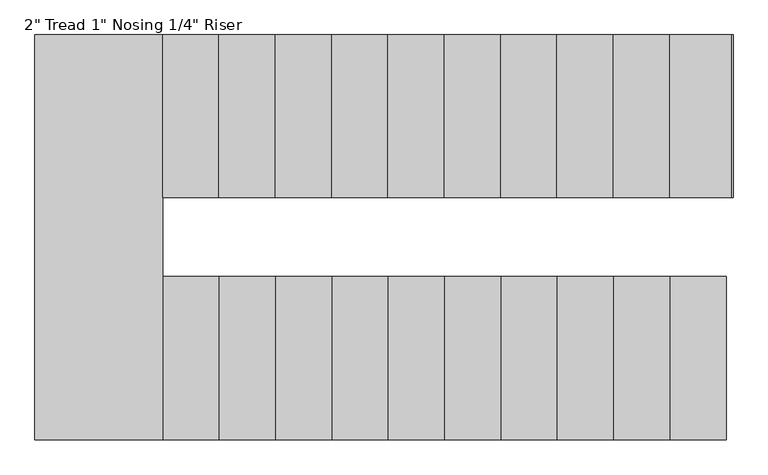
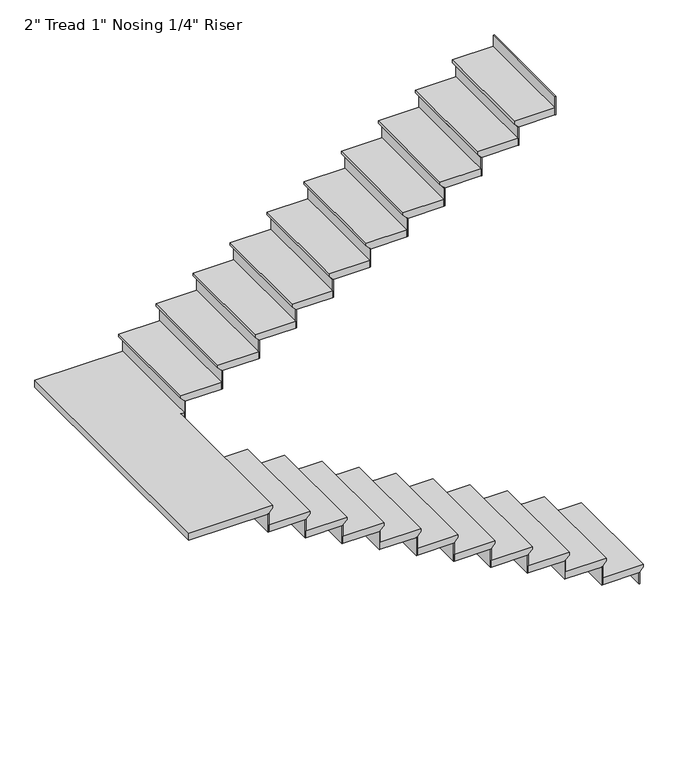
"""IFC4 building model written with IfcOpenShell, lengths in millimetres: stair flight geometry."""

from ifc_helpers import new_model, si_unit, origin, place, context, project, spatial, faceted_brep, source, transform, mapped, element, save


def stair_flight_f3bed003(model_context):
    return source(origin(), model_context, "Body", "Brep", [
        faceted_brep([(-3117.2664982, -6914.3822004, 112.5681818), (-3117.2664982, -6914.3822004, 131.6181818), (-3117.2664982, -7650.9822004, 131.6181818), (-3117.2664982, -7650.9822004, 112.5681818), (-3142.6664982, -6914.3822004, 87.1681818), (-3142.6664982, -7650.9822004, 87.1681818), (-3396.6664982, -6914.3822004, 131.6181818), (-3396.6664982, -7650.9822004, 131.6181818), (-3142.6664982, -7650.9822004, 80.8181818), (-3396.6664982, -7650.9822004, 80.8181818), (-3396.6664982, -6914.3822004, 80.8181818), (-3142.6664982, -6914.3822004, 80.8181818)], [[[0, 1, 2, 3]], [[4, 0, 3, 5]], [[2, 1, 6, 7]], [[8, 9, 10, 11]], [[2, 7, 9, 8, 5, 3]], [[8, 11, 4, 5]], [[6, 1, 0, 4, 11, 10]], [[7, 6, 10, 9]]]),
        faceted_brep([(-3142.6664982, -6914.3822004, 80.8181818), (-3142.6664982, -6914.3822004, 0.0), (-3149.0164982, -6914.3822004, 0.0), (-3149.0164982, -6914.3822004, 80.8181818), (-3142.6664982, -7650.9822004, 80.8181818), (-3149.0164982, -7650.9822004, 80.8181818), (-3149.0164982, -7650.9822004, 0.0), (-3142.6664982, -7650.9822004, 0.0)], [[[0, 1, 2, 3]], [[4, 5, 6, 7]], [[1, 0, 4, 7]], [[2, 1, 7, 6]], [[3, 2, 6, 5]], [[0, 3, 5, 4]]]),
        faceted_brep([(-3396.6664982, -6914.3822004, 212.4363636), (-3396.6664982, -6914.3822004, 80.8181818), (-3403.0164982, -6914.3822004, 80.8181818), (-3403.0164982, -6914.3822004, 212.4363636), (-3396.6664982, -7650.9822004, 212.4363636), (-3403.0164982, -7650.9822004, 212.4363636), (-3403.0164982, -7650.9822004, 80.8181818), (-3396.6664982, -7650.9822004, 80.8181818)], [[[0, 1, 2, 3]], [[4, 5, 6, 7]], [[1, 0, 4, 7]], [[2, 1, 7, 6]], [[3, 2, 6, 5]], [[0, 3, 5, 4]]]),
        faceted_brep([(-3371.2664982, -7650.9822004, 263.2363636), (-3371.2664982, -6914.3822004, 263.2363636), (-3650.6664982, -6914.3822004, 263.2363636), (-3650.6664982, -7650.9822004, 263.2363636), (-3396.6664982, -7650.9822004, 212.4363636), (-3650.6664982, -7650.9822004, 212.4363636), (-3650.6664982, -6914.3822004, 212.4363636), (-3396.6664982, -6914.3822004, 212.4363636), (-3396.6664982, -7650.9822004, 218.7863636), (-3371.2664982, -7650.9822004, 244.1863636), (-3396.6664982, -6914.3822004, 218.7863636), (-3371.2664982, -6914.3822004, 244.1863636)], [[[0, 1, 2, 3]], [[4, 5, 6, 7]], [[0, 3, 5, 4, 8, 9]], [[4, 7, 10, 8]], [[2, 1, 11, 10, 7, 6]], [[3, 2, 6, 5]], [[11, 1, 0, 9]], [[10, 11, 9, 8]]]),
        faceted_brep([(-3650.6664982, -6914.3822004, 344.0545455), (-3650.6664982, -6914.3822004, 212.4363636), (-3657.0164982, -6914.3822004, 212.4363636), (-3657.0164982, -6914.3822004, 344.0545455), (-3650.6664982, -7650.9822004, 344.0545455), (-3657.0164982, -7650.9822004, 344.0545455), (-3657.0164982, -7650.9822004, 212.4363636), (-3650.6664982, -7650.9822004, 212.4363636)], [[[0, 1, 2, 3]], [[4, 5, 6, 7]], [[1, 0, 4, 7]], [[2, 1, 7, 6]], [[3, 2, 6, 5]], [[0, 3, 5, 4]]]),
        faceted_brep([(-3625.2664982, -7650.9822004, 394.8545455), (-3625.2664982, -6914.3822004, 394.8545455), (-3904.6664982, -6914.3822004, 394.8545455), (-3904.6664982, -7650.9822004, 394.8545455), (-3650.6664982, -7650.9822004, 344.0545455), (-3904.6664982, -7650.9822004, 344.0545455), (-3904.6664982, -6914.3822004, 344.0545455), (-3650.6664982, -6914.3822004, 344.0545455), (-3650.6664982, -7650.9822004, 350.4045455), (-3625.2664982, -7650.9822004, 375.8045455), (-3650.6664982, -6914.3822004, 350.4045455), (-3625.2664982, -6914.3822004, 375.8045455)], [[[0, 1, 2, 3]], [[4, 5, 6, 7]], [[0, 3, 5, 4, 8, 9]], [[4, 7, 10, 8]], [[2, 1, 11, 10, 7, 6]], [[3, 2, 6, 5]], [[11, 1, 0, 9]], [[10, 11, 9, 8]]]),
        faceted_brep([(-3904.6664982, -6914.3822004, 475.6727273), (-3904.6664982, -6914.3822004, 344.0545455), (-3911.0164982, -6914.3822004, 344.0545455), (-3911.0164982, -6914.3822004, 475.6727273), (-3904.6664982, -7650.9822004, 475.6727273), (-3911.0164982, -7650.9822004, 475.6727273), (-3911.0164982, -7650.9822004, 344.0545455), (-3904.6664982, -7650.9822004, 344.0545455)], [[[0, 1, 2, 3]], [[4, 5, 6, 7]], [[1, 0, 4, 7]], [[2, 1, 7, 6]], [[3, 2, 6, 5]], [[0, 3, 5, 4]]]),
        faceted_brep([(-3879.2664982, -7650.9822004, 526.4727273), (-3879.2664982, -6914.3822004, 526.4727273), (-4158.6664982, -6914.3822004, 526.4727273), (-4158.6664982, -7650.9822004, 526.4727273), (-3904.6664982, -7650.9822004, 475.6727273), (-4158.6664982, -7650.9822004, 475.6727273), (-4158.6664982, -6914.3822004, 475.6727273), (-3904.6664982, -6914.3822004, 475.6727273), (-3904.6664982, -7650.9822004, 482.0227273), (-3879.2664982, -7650.9822004, 507.4227273), (-3904.6664982, -6914.3822004, 482.0227273), (-3879.2664982, -6914.3822004, 507.4227273)], [[[0, 1, 2, 3]], [[4, 5, 6, 7]], [[0, 3, 5, 4, 8, 9]], [[4, 7, 10, 8]], [[2, 1, 11, 10, 7, 6]], [[3, 2, 6, 5]], [[11, 1, 0, 9]], [[10, 11, 9, 8]]]),
        faceted_brep([(-4158.6664982, -6914.3822004, 607.2909091), (-4158.6664982, -6914.3822004, 475.6727273), (-4165.0164982, -6914.3822004, 475.6727273), (-4165.0164982, -6914.3822004, 607.2909091), (-4158.6664982, -7650.9822004, 607.2909091), (-4165.0164982, -7650.9822004, 607.2909091), (-4165.0164982, -7650.9822004, 475.6727273), (-4158.6664982, -7650.9822004, 475.6727273)], [[[0, 1, 2, 3]], [[4, 5, 6, 7]], [[1, 0, 4, 7]], [[2, 1, 7, 6]], [[3, 2, 6, 5]], [[0, 3, 5, 4]]]),
        faceted_brep([(-4133.2664982, -7650.9822004, 658.0909091), (-4133.2664982, -6914.3822004, 658.0909091), (-4412.6664982, -6914.3822004, 658.0909091), (-4412.6664982, -7650.9822004, 658.0909091), (-4158.6664982, -7650.9822004, 607.2909091), (-4412.6664982, -7650.9822004, 607.2909091), (-4412.6664982, -6914.3822004, 607.2909091), (-4158.6664982, -6914.3822004, 607.2909091), (-4158.6664982, -7650.9822004, 613.6409091), (-4133.2664982, -7650.9822004, 639.0409091), (-4158.6664982, -6914.3822004, 613.6409091), (-4133.2664982, -6914.3822004, 639.0409091)], [[[0, 1, 2, 3]], [[4, 5, 6, 7]], [[0, 3, 5, 4, 8, 9]], [[4, 7, 10, 8]], [[2, 1, 11, 10, 7, 6]], [[3, 2, 6, 5]], [[11, 1, 0, 9]], [[10, 11, 9, 8]]]),
        faceted_brep([(-4412.6664982, -6914.3822004, 738.9090909), (-4412.6664982, -6914.3822004, 607.2909091), (-4419.0164982, -6914.3822004, 607.2909091), (-4419.0164982, -6914.3822004, 738.9090909), (-4412.6664982, -7650.9822004, 738.9090909), (-4419.0164982, -7650.9822004, 738.9090909), (-4419.0164982, -7650.9822004, 607.2909091), (-4412.6664982, -7650.9822004, 607.2909091)], [[[0, 1, 2, 3]], [[4, 5, 6, 7]], [[1, 0, 4, 7]], [[2, 1, 7, 6]], [[3, 2, 6, 5]], [[0, 3, 5, 4]]]),
        faceted_brep([(-4387.2664982, -7650.9822004, 789.7090909), (-4387.2664982, -6914.3822004, 789.7090909), (-4666.6664982, -6914.3822004, 789.7090909), (-4666.6664982, -7650.9822004, 789.7090909), (-4412.6664982, -7650.9822004, 738.9090909), (-4666.6664982, -7650.9822004, 738.9090909), (-4666.6664982, -6914.3822004, 738.9090909), (-4412.6664982, -6914.3822004, 738.9090909), (-4412.6664982, -7650.9822004, 745.2590909), (-4387.2664982, -7650.9822004, 770.6590909), (-4412.6664982, -6914.3822004, 745.2590909), (-4387.2664982, -6914.3822004, 770.6590909)], [[[0, 1, 2, 3]], [[4, 5, 6, 7]], [[0, 3, 5, 4, 8, 9]], [[4, 7, 10, 8]], [[2, 1, 11, 10, 7, 6]], [[3, 2, 6, 5]], [[11, 1, 0, 9]], [[10, 11, 9, 8]]]),
        faceted_brep([(-4666.6664982, -6914.3822004, 870.5272727), (-4666.6664982, -6914.3822004, 738.9090909), (-4673.0164982, -6914.3822004, 738.9090909), (-4673.0164982, -6914.3822004, 870.5272727), (-4666.6664982, -7650.9822004, 870.5272727), (-4673.0164982, -7650.9822004, 870.5272727), (-4673.0164982, -7650.9822004, 738.9090909), (-4666.6664982, -7650.9822004, 738.9090909)], [[[0, 1, 2, 3]], [[4, 5, 6, 7]], [[1, 0, 4, 7]], [[2, 1, 7, 6]], [[3, 2, 6, 5]], [[0, 3, 5, 4]]]),
        faceted_brep([(-4641.2664982, -7650.9822004, 921.3272727), (-4641.2664982, -6914.3822004, 921.3272727), (-4920.6664982, -6914.3822004, 921.3272727), (-4920.6664982, -7650.9822004, 921.3272727), (-4666.6664982, -7650.9822004, 870.5272727), (-4920.6664982, -7650.9822004, 870.5272727), (-4920.6664982, -6914.3822004, 870.5272727), (-4666.6664982, -6914.3822004, 870.5272727), (-4666.6664982, -7650.9822004, 876.8772727), (-4641.2664982, -7650.9822004, 902.2772727), (-4666.6664982, -6914.3822004, 876.8772727), (-4641.2664982, -6914.3822004, 902.2772727)], [[[0, 1, 2, 3]], [[4, 5, 6, 7]], [[0, 3, 5, 4, 8, 9]], [[4, 7, 10, 8]], [[2, 1, 11, 10, 7, 6]], [[3, 2, 6, 5]], [[11, 1, 0, 9]], [[10, 11, 9, 8]]]),
        faceted_brep([(-4920.6664982, -6914.3822004, 1002.1454545), (-4920.6664982, -6914.3822004, 870.5272727), (-4927.0164982, -6914.3822004, 870.5272727), (-4927.0164982, -6914.3822004, 1002.1454545), (-4920.6664982, -7650.9822004, 1002.1454545), (-4927.0164982, -7650.9822004, 1002.1454545), (-4927.0164982, -7650.9822004, 870.5272727), (-4920.6664982, -7650.9822004, 870.5272727)], [[[0, 1, 2, 3]], [[4, 5, 6, 7]], [[1, 0, 4, 7]], [[2, 1, 7, 6]], [[3, 2, 6, 5]], [[0, 3, 5, 4]]]),
        faceted_brep([(-4895.2664982, -7650.9822004, 1052.9454545), (-4895.2664982, -6914.3822004, 1052.9454545), (-5174.6664982, -6914.3822004, 1052.9454545), (-5174.6664982, -7650.9822004, 1052.9454545), (-4920.6664982, -7650.9822004, 1002.1454545), (-5174.6664982, -7650.9822004, 1002.1454545), (-5174.6664982, -6914.3822004, 1002.1454545), (-4920.6664982, -6914.3822004, 1002.1454545), (-4920.6664982, -7650.9822004, 1008.4954545), (-4895.2664982, -7650.9822004, 1033.8954545), (-4920.6664982, -6914.3822004, 1008.4954545), (-4895.2664982, -6914.3822004, 1033.8954545)], [[[0, 1, 2, 3]], [[4, 5, 6, 7]], [[0, 3, 5, 4, 8, 9]], [[4, 7, 10, 8]], [[2, 1, 11, 10, 7, 6]], [[3, 2, 6, 5]], [[11, 1, 0, 9]], [[10, 11, 9, 8]]]),
        faceted_brep([(-5174.6664982, -6914.3822004, 1133.7636364), (-5174.6664982, -6914.3822004, 1002.1454545), (-5181.0164982, -6914.3822004, 1002.1454545), (-5181.0164982, -6914.3822004, 1133.7636364), (-5174.6664982, -7650.9822004, 1133.7636364), (-5181.0164982, -7650.9822004, 1133.7636364), (-5181.0164982, -7650.9822004, 1002.1454545), (-5174.6664982, -7650.9822004, 1002.1454545)], [[[0, 1, 2, 3]], [[4, 5, 6, 7]], [[1, 0, 4, 7]], [[2, 1, 7, 6]], [[3, 2, 6, 5]], [[0, 3, 5, 4]]]),
        faceted_brep([(-5149.2664982, -7650.9822004, 1184.5636364), (-5149.2664982, -6914.3822004, 1184.5636364), (-5428.6664982, -6914.3822004, 1184.5636364), (-5428.6664982, -7650.9822004, 1184.5636364), (-5174.6664982, -7650.9822004, 1133.7636364), (-5428.6664982, -7650.9822004, 1133.7636364), (-5428.6664982, -6914.3822004, 1133.7636364), (-5174.6664982, -6914.3822004, 1133.7636364), (-5174.6664982, -7650.9822004, 1140.1136364), (-5149.2664982, -7650.9822004, 1165.5136364), (-5174.6664982, -6914.3822004, 1140.1136364), (-5149.2664982, -6914.3822004, 1165.5136364)], [[[0, 1, 2, 3]], [[4, 5, 6, 7]], [[0, 3, 5, 4, 8, 9]], [[4, 7, 10, 8]], [[2, 1, 11, 10, 7, 6]], [[3, 2, 6, 5]], [[11, 1, 0, 9]], [[10, 11, 9, 8]]]),
        faceted_brep([(-5428.6664982, -6914.3822004, 1265.3818182), (-5428.6664982, -6914.3822004, 1133.7636364), (-5435.0164982, -6914.3822004, 1133.7636364), (-5435.0164982, -6914.3822004, 1265.3818182), (-5428.6664982, -7650.9822004, 1265.3818182), (-5435.0164982, -7650.9822004, 1265.3818182), (-5435.0164982, -7650.9822004, 1133.7636364), (-5428.6664982, -7650.9822004, 1133.7636364)], [[[0, 1, 2, 3]], [[4, 5, 6, 7]], [[1, 0, 4, 7]], [[2, 1, 7, 6]], [[3, 2, 6, 5]], [[0, 3, 5, 4]]]),
        faceted_brep([(-5403.2664982, -7650.9822004, 1316.1818182), (-5403.2664982, -6914.3822004, 1316.1818182), (-5682.6664982, -6914.3822004, 1316.1818182), (-5682.6664982, -7650.9822004, 1316.1818182), (-5428.6664982, -7650.9822004, 1265.3818182), (-5682.6664982, -7650.9822004, 1265.3818182), (-5682.6664982, -6914.3822004, 1265.3818182), (-5428.6664982, -6914.3822004, 1265.3818182), (-5428.6664982, -7650.9822004, 1271.7318182), (-5403.2664982, -7650.9822004, 1297.1318182), (-5428.6664982, -6914.3822004, 1271.7318182), (-5403.2664982, -6914.3822004, 1297.1318182)], [[[0, 1, 2, 3]], [[4, 5, 6, 7]], [[0, 3, 5, 4, 8, 9]], [[4, 7, 10, 8]], [[2, 1, 11, 10, 7, 6]], [[3, 2, 6, 5]], [[11, 1, 0, 9]], [[10, 11, 9, 8]]]),
        faceted_brep([(-5682.6664982, -6914.3822004, 1397.0), (-5682.6664982, -6914.3822004, 1265.3818182), (-5689.0164982, -6914.3822004, 1265.3818182), (-5689.0164982, -6914.3822004, 1397.0), (-5682.6664982, -7650.9822004, 1397.0), (-5689.0164982, -7650.9822004, 1397.0), (-5689.0164982, -7650.9822004, 1265.3818182), (-5682.6664982, -7650.9822004, 1265.3818182)], [[[0, 1, 2, 3]], [[4, 5, 6, 7]], [[1, 0, 4, 7]], [[2, 1, 7, 6]], [[3, 2, 6, 5]], [[0, 3, 5, 4]]]),
        faceted_brep([(-5631.8664982, -5824.7082131, 1447.8), (-6232.5131972, -5824.7082131, 1447.8), (-6232.5131972, -7650.9822004, 1447.8), (-5657.2664982, -7650.9822004, 1447.8), (-5657.2664982, -6558.7822004, 1447.8), (-5631.8664982, -6558.7822004, 1447.8), (-6232.5131972, -5824.7082131, 1397.0), (-5631.8664982, -5824.7082131, 1397.0), (-5631.8664982, -6558.7822004, 1397.0), (-5657.2664982, -6558.7822004, 1397.0), (-5657.2664982, -6914.3822004, 1397.0), (-5682.6664982, -6914.3822004, 1397.0), (-5682.6664982, -7650.9822004, 1397.0), (-6232.5131972, -7650.9822004, 1397.0), (-5682.6664982, -6914.3822004, 1403.35), (-5682.6664982, -7650.9822004, 1403.35), (-5657.2664982, -7650.9822004, 1428.75), (-5657.2664982, -6914.3822004, 1428.75)], [[[0, 1, 2, 3, 4, 5]], [[6, 7, 8, 9, 10, 11, 12, 13]], [[1, 0, 7, 6]], [[2, 1, 6, 13]], [[12, 11, 14, 15]], [[4, 3, 16, 17, 10, 9]], [[5, 4, 9, 8]], [[0, 5, 8, 7]], [[16, 15, 14, 17]], [[3, 2, 13, 12, 15, 16]], [[11, 10, 17, 14]]]),
        faceted_brep([(-5631.8664982, -6558.7822004, 1528.6181818), (-5631.8664982, -6558.7822004, 1397.0), (-5625.5164982, -6558.7822004, 1397.0), (-5625.5164982, -6558.7822004, 1528.6181818), (-5631.8664982, -5824.7082131, 1528.6181818), (-5625.5164982, -5824.7082131, 1528.6181818), (-5625.5164982, -5824.7082131, 1397.0), (-5631.8664982, -5824.7082131, 1397.0)], [[[0, 1, 2, 3]], [[4, 5, 6, 7]], [[1, 0, 4, 7]], [[2, 1, 7, 6]], [[3, 2, 6, 5]], [[0, 3, 5, 4]]]),
        faceted_brep([(-5657.2664982, -5824.7082131, 1579.4181818), (-5657.2664982, -6558.7822004, 1579.4181818), (-5377.8664982, -6558.7822004, 1579.4181818), (-5377.8664982, -5824.7082131, 1579.4181818), (-5631.8664982, -5824.7082131, 1528.6181818), (-5377.8664982, -5824.7082131, 1528.6181818), (-5377.8664982, -6558.7822004, 1528.6181818), (-5631.8664982, -6558.7822004, 1528.6181818), (-5631.8664982, -5824.7082131, 1534.9681818), (-5657.2664982, -5824.7082131, 1560.3681818), (-5631.8664982, -6558.7822004, 1534.9681818), (-5657.2664982, -6558.7822004, 1560.3681818)], [[[0, 1, 2, 3]], [[4, 5, 6, 7]], [[0, 3, 5, 4, 8, 9]], [[4, 7, 10, 8]], [[2, 1, 11, 10, 7, 6]], [[3, 2, 6, 5]], [[11, 1, 0, 9]], [[10, 11, 9, 8]]]),
        faceted_brep([(-5377.8664982, -6558.7822004, 1660.2363636), (-5377.8664982, -6558.7822004, 1528.6181818), (-5371.5164982, -6558.7822004, 1528.6181818), (-5371.5164982, -6558.7822004, 1660.2363636), (-5377.8664982, -5824.7082131, 1660.2363636), (-5371.5164982, -5824.7082131, 1660.2363636), (-5371.5164982, -5824.7082131, 1528.6181818), (-5377.8664982, -5824.7082131, 1528.6181818)], [[[0, 1, 2, 3]], [[4, 5, 6, 7]], [[1, 0, 4, 7]], [[2, 1, 7, 6]], [[3, 2, 6, 5]], [[0, 3, 5, 4]]]),
        faceted_brep([(-5403.2664982, -5824.7082131, 1711.0363636), (-5403.2664982, -6558.7822004, 1711.0363636), (-5123.8664982, -6558.7822004, 1711.0363636), (-5123.8664982, -5824.7082131, 1711.0363636), (-5377.8664982, -5824.7082131, 1660.2363636), (-5123.8664982, -5824.7082131, 1660.2363636), (-5123.8664982, -6558.7822004, 1660.2363636), (-5377.8664982, -6558.7822004, 1660.2363636), (-5377.8664982, -5824.7082131, 1666.5863636), (-5403.2664982, -5824.7082131, 1691.9863636), (-5377.8664982, -6558.7822004, 1666.5863636), (-5403.2664982, -6558.7822004, 1691.9863636)], [[[0, 1, 2, 3]], [[4, 5, 6, 7]], [[0, 3, 5, 4, 8, 9]], [[4, 7, 10, 8]], [[2, 1, 11, 10, 7, 6]], [[3, 2, 6, 5]], [[11, 1, 0, 9]], [[10, 11, 9, 8]]]),
        faceted_brep([(-5123.8664982, -6558.7822004, 1791.8545455), (-5123.8664982, -6558.7822004, 1660.2363636), (-5117.5164982, -6558.7822004, 1660.2363636), (-5117.5164982, -6558.7822004, 1791.8545455), (-5123.8664982, -5824.7082131, 1791.8545455), (-5117.5164982, -5824.7082131, 1791.8545455), (-5117.5164982, -5824.7082131, 1660.2363636), (-5123.8664982, -5824.7082131, 1660.2363636)], [[[0, 1, 2, 3]], [[4, 5, 6, 7]], [[1, 0, 4, 7]], [[2, 1, 7, 6]], [[3, 2, 6, 5]], [[0, 3, 5, 4]]]),
        faceted_brep([(-5149.2664982, -5824.7082131, 1842.6545455), (-5149.2664982, -6558.7822004, 1842.6545455), (-4869.8664982, -6558.7822004, 1842.6545455), (-4869.8664982, -5824.7082131, 1842.6545455), (-5123.8664982, -5824.7082131, 1791.8545455), (-4869.8664982, -5824.7082131, 1791.8545455), (-4869.8664982, -6558.7822004, 1791.8545455), (-5123.8664982, -6558.7822004, 1791.8545455), (-5123.8664982, -5824.7082131, 1798.2045455), (-5149.2664982, -5824.7082131, 1823.6045455), (-5123.8664982, -6558.7822004, 1798.2045455), (-5149.2664982, -6558.7822004, 1823.6045455)], [[[0, 1, 2, 3]], [[4, 5, 6, 7]], [[0, 3, 5, 4, 8, 9]], [[4, 7, 10, 8]], [[2, 1, 11, 10, 7, 6]], [[3, 2, 6, 5]], [[11, 1, 0, 9]], [[10, 11, 9, 8]]]),
        faceted_brep([(-4869.8664982, -6558.7822004, 1923.4727273), (-4869.8664982, -6558.7822004, 1791.8545455), (-4863.5164982, -6558.7822004, 1791.8545455), (-4863.5164982, -6558.7822004, 1923.4727273), (-4869.8664982, -5824.7082131, 1923.4727273), (-4863.5164982, -5824.7082131, 1923.4727273), (-4863.5164982, -5824.7082131, 1791.8545455), (-4869.8664982, -5824.7082131, 1791.8545455)], [[[0, 1, 2, 3]], [[4, 5, 6, 7]], [[1, 0, 4, 7]], [[2, 1, 7, 6]], [[3, 2, 6, 5]], [[0, 3, 5, 4]]]),
        faceted_brep([(-4895.2664982, -5824.7082131, 1974.2727273), (-4895.2664982, -6558.7822004, 1974.2727273), (-4615.8664982, -6558.7822004, 1974.2727273), (-4615.8664982, -5824.7082131, 1974.2727273), (-4869.8664982, -5824.7082131, 1923.4727273), (-4615.8664982, -5824.7082131, 1923.4727273), (-4615.8664982, -6558.7822004, 1923.4727273), (-4869.8664982, -6558.7822004, 1923.4727273), (-4869.8664982, -5824.7082131, 1929.8227273), (-4895.2664982, -5824.7082131, 1955.2227273), (-4869.8664982, -6558.7822004, 1929.8227273), (-4895.2664982, -6558.7822004, 1955.2227273)], [[[0, 1, 2, 3]], [[4, 5, 6, 7]], [[0, 3, 5, 4, 8, 9]], [[4, 7, 10, 8]], [[2, 1, 11, 10, 7, 6]], [[3, 2, 6, 5]], [[11, 1, 0, 9]], [[10, 11, 9, 8]]]),
        faceted_brep([(-4615.8664982, -6558.7822004, 2055.0909091), (-4615.8664982, -6558.7822004, 1923.4727273), (-4609.5164982, -6558.7822004, 1923.4727273), (-4609.5164982, -6558.7822004, 2055.0909091), (-4615.8664982, -5824.7082131, 2055.0909091), (-4609.5164982, -5824.7082131, 2055.0909091), (-4609.5164982, -5824.7082131, 1923.4727273), (-4615.8664982, -5824.7082131, 1923.4727273)], [[[0, 1, 2, 3]], [[4, 5, 6, 7]], [[1, 0, 4, 7]], [[2, 1, 7, 6]], [[3, 2, 6, 5]], [[0, 3, 5, 4]]]),
        faceted_brep([(-4641.2664982, -5824.7082131, 2105.8909091), (-4641.2664982, -6558.7822004, 2105.8909091), (-4361.8664982, -6558.7822004, 2105.8909091), (-4361.8664982, -5824.7082131, 2105.8909091), (-4615.8664982, -5824.7082131, 2055.0909091), (-4361.8664982, -5824.7082131, 2055.0909091), (-4361.8664982, -6558.7822004, 2055.0909091), (-4615.8664982, -6558.7822004, 2055.0909091), (-4615.8664982, -5824.7082131, 2061.4409091), (-4641.2664982, -5824.7082131, 2086.8409091), (-4615.8664982, -6558.7822004, 2061.4409091), (-4641.2664982, -6558.7822004, 2086.8409091)], [[[0, 1, 2, 3]], [[4, 5, 6, 7]], [[0, 3, 5, 4, 8, 9]], [[4, 7, 10, 8]], [[2, 1, 11, 10, 7, 6]], [[3, 2, 6, 5]], [[11, 1, 0, 9]], [[10, 11, 9, 8]]]),
        faceted_brep([(-4361.8664982, -6558.7822004, 2186.7090909), (-4361.8664982, -6558.7822004, 2055.0909091), (-4355.5164982, -6558.7822004, 2055.0909091), (-4355.5164982, -6558.7822004, 2186.7090909), (-4361.8664982, -5824.7082131, 2186.7090909), (-4355.5164982, -5824.7082131, 2186.7090909), (-4355.5164982, -5824.7082131, 2055.0909091), (-4361.8664982, -5824.7082131, 2055.0909091)], [[[0, 1, 2, 3]], [[4, 5, 6, 7]], [[1, 0, 4, 7]], [[2, 1, 7, 6]], [[3, 2, 6, 5]], [[0, 3, 5, 4]]]),
        faceted_brep([(-4387.2664982, -5824.7082131, 2237.5090909), (-4387.2664982, -6558.7822004, 2237.5090909), (-4107.8664982, -6558.7822004, 2237.5090909), (-4107.8664982, -5824.7082131, 2237.5090909), (-4361.8664982, -5824.7082131, 2186.7090909), (-4107.8664982, -5824.7082131, 2186.7090909), (-4107.8664982, -6558.7822004, 2186.7090909), (-4361.8664982, -6558.7822004, 2186.7090909), (-4361.8664982, -5824.7082131, 2193.0590909), (-4387.2664982, -5824.7082131, 2218.4590909), (-4361.8664982, -6558.7822004, 2193.0590909), (-4387.2664982, -6558.7822004, 2218.4590909)], [[[0, 1, 2, 3]], [[4, 5, 6, 7]], [[0, 3, 5, 4, 8, 9]], [[4, 7, 10, 8]], [[2, 1, 11, 10, 7, 6]], [[3, 2, 6, 5]], [[11, 1, 0, 9]], [[10, 11, 9, 8]]]),
        faceted_brep([(-4107.8664982, -6558.7822004, 2318.3272727), (-4107.8664982, -6558.7822004, 2186.7090909), (-4101.5164982, -6558.7822004, 2186.7090909), (-4101.5164982, -6558.7822004, 2318.3272727), (-4107.8664982, -5824.7082131, 2318.3272727), (-4101.5164982, -5824.7082131, 2318.3272727), (-4101.5164982, -5824.7082131, 2186.7090909), (-4107.8664982, -5824.7082131, 2186.7090909)], [[[0, 1, 2, 3]], [[4, 5, 6, 7]], [[1, 0, 4, 7]], [[2, 1, 7, 6]], [[3, 2, 6, 5]], [[0, 3, 5, 4]]]),
        faceted_brep([(-4133.2664982, -5824.7082131, 2369.1272727), (-4133.2664982, -6558.7822004, 2369.1272727), (-3853.8664982, -6558.7822004, 2369.1272727), (-3853.8664982, -5824.7082131, 2369.1272727), (-4107.8664982, -5824.7082131, 2318.3272727), (-3853.8664982, -5824.7082131, 2318.3272727), (-3853.8664982, -6558.7822004, 2318.3272727), (-4107.8664982, -6558.7822004, 2318.3272727), (-4107.8664982, -5824.7082131, 2324.6772727), (-4133.2664982, -5824.7082131, 2350.0772727), (-4107.8664982, -6558.7822004, 2324.6772727), (-4133.2664982, -6558.7822004, 2350.0772727)], [[[0, 1, 2, 3]], [[4, 5, 6, 7]], [[0, 3, 5, 4, 8, 9]], [[4, 7, 10, 8]], [[2, 1, 11, 10, 7, 6]], [[3, 2, 6, 5]], [[11, 1, 0, 9]], [[10, 11, 9, 8]]]),
        faceted_brep([(-3853.8664982, -6558.7822004, 2449.9454545), (-3853.8664982, -6558.7822004, 2318.3272727), (-3847.5164982, -6558.7822004, 2318.3272727), (-3847.5164982, -6558.7822004, 2449.9454545), (-3853.8664982, -5824.7082131, 2449.9454545), (-3847.5164982, -5824.7082131, 2449.9454545), (-3847.5164982, -5824.7082131, 2318.3272727), (-3853.8664982, -5824.7082131, 2318.3272727)], [[[0, 1, 2, 3]], [[4, 5, 6, 7]], [[1, 0, 4, 7]], [[2, 1, 7, 6]], [[3, 2, 6, 5]], [[0, 3, 5, 4]]]),
        faceted_brep([(-3879.2664982, -5824.7082131, 2500.7454545), (-3879.2664982, -6558.7822004, 2500.7454545), (-3599.8664982, -6558.7822004, 2500.7454545), (-3599.8664982, -5824.7082131, 2500.7454545), (-3853.8664982, -5824.7082131, 2449.9454545), (-3599.8664982, -5824.7082131, 2449.9454545), (-3599.8664982, -6558.7822004, 2449.9454545), (-3853.8664982, -6558.7822004, 2449.9454545), (-3853.8664982, -5824.7082131, 2456.2954545), (-3879.2664982, -5824.7082131, 2481.6954545), (-3853.8664982, -6558.7822004, 2456.2954545), (-3879.2664982, -6558.7822004, 2481.6954545)], [[[0, 1, 2, 3]], [[4, 5, 6, 7]], [[0, 3, 5, 4, 8, 9]], [[4, 7, 10, 8]], [[2, 1, 11, 10, 7, 6]], [[3, 2, 6, 5]], [[11, 1, 0, 9]], [[10, 11, 9, 8]]]),
        faceted_brep([(-3599.8664982, -6558.7822004, 2581.5636364), (-3599.8664982, -6558.7822004, 2449.9454545), (-3593.5164982, -6558.7822004, 2449.9454545), (-3593.5164982, -6558.7822004, 2581.5636364), (-3599.8664982, -5824.7082131, 2581.5636364), (-3593.5164982, -5824.7082131, 2581.5636364), (-3593.5164982, -5824.7082131, 2449.9454545), (-3599.8664982, -5824.7082131, 2449.9454545)], [[[0, 1, 2, 3]], [[4, 5, 6, 7]], [[1, 0, 4, 7]], [[2, 1, 7, 6]], [[3, 2, 6, 5]], [[0, 3, 5, 4]]]),
        faceted_brep([(-3625.2664982, -5824.7082131, 2632.3636364), (-3625.2664982, -6558.7822004, 2632.3636364), (-3345.8664982, -6558.7822004, 2632.3636364), (-3345.8664982, -5824.7082131, 2632.3636364), (-3599.8664982, -5824.7082131, 2581.5636364), (-3345.8664982, -5824.7082131, 2581.5636364), (-3345.8664982, -6558.7822004, 2581.5636364), (-3599.8664982, -6558.7822004, 2581.5636364), (-3599.8664982, -5824.7082131, 2587.9136364), (-3625.2664982, -5824.7082131, 2613.3136364), (-3599.8664982, -6558.7822004, 2587.9136364), (-3625.2664982, -6558.7822004, 2613.3136364)], [[[0, 1, 2, 3]], [[4, 5, 6, 7]], [[0, 3, 5, 4, 8, 9]], [[4, 7, 10, 8]], [[2, 1, 11, 10, 7, 6]], [[3, 2, 6, 5]], [[11, 1, 0, 9]], [[10, 11, 9, 8]]]),
        faceted_brep([(-3345.8664982, -6558.7822004, 2713.1818182), (-3345.8664982, -6558.7822004, 2581.5636364), (-3339.5164982, -6558.7822004, 2581.5636364), (-3339.5164982, -6558.7822004, 2713.1818182), (-3345.8664982, -5824.7082131, 2713.1818182), (-3339.5164982, -5824.7082131, 2713.1818182), (-3339.5164982, -5824.7082131, 2581.5636364), (-3345.8664982, -5824.7082131, 2581.5636364)], [[[0, 1, 2, 3]], [[4, 5, 6, 7]], [[1, 0, 4, 7]], [[2, 1, 7, 6]], [[3, 2, 6, 5]], [[0, 3, 5, 4]]]),
        faceted_brep([(-3091.8664982, -6558.7822004, 2844.8), (-3091.8664982, -6558.7822004, 2713.1818182), (-3085.5164982, -6558.7822004, 2713.1818182), (-3085.5164982, -6558.7822004, 2844.8), (-3091.8664982, -5824.7082131, 2844.8), (-3085.5164982, -5824.7082131, 2844.8), (-3085.5164982, -5824.7082131, 2713.1818182), (-3091.8664982, -5824.7082131, 2713.1818182)], [[[0, 1, 2, 3]], [[4, 5, 6, 7]], [[1, 0, 4, 7]], [[2, 1, 7, 6]], [[3, 2, 6, 5]], [[0, 3, 5, 4]]]),
        faceted_brep([(-3371.2664982, -5824.7082131, 2763.9818182), (-3371.2664982, -6558.7822004, 2763.9818182), (-3091.8664982, -6558.7822004, 2763.9818182), (-3091.8664982, -5824.7082131, 2763.9818182), (-3345.8664982, -5824.7082131, 2713.1818182), (-3091.8664982, -5824.7082131, 2713.1818182), (-3091.8664982, -6558.7822004, 2713.1818182), (-3345.8664982, -6558.7822004, 2713.1818182), (-3345.8664982, -5824.7082131, 2719.5318182), (-3371.2664982, -5824.7082131, 2744.9318182), (-3345.8664982, -6558.7822004, 2719.5318182), (-3371.2664982, -6558.7822004, 2744.9318182)], [[[0, 1, 2, 3]], [[4, 5, 6, 7]], [[0, 3, 5, 4, 8, 9]], [[4, 7, 10, 8]], [[2, 1, 11, 10, 7, 6]], [[3, 2, 6, 5]], [[11, 1, 0, 9]], [[10, 11, 9, 8]]]),
    ])


if __name__ == "__main__":
    model = new_model("IFC4")
    model_context = context("Model", 3, world=origin())
    ifc_project = project(units=[si_unit("LENGTHUNIT", "METRE", prefix="MILLI")], contexts=[model_context])
    site = spatial("IfcSite", under=ifc_project)
    building = spatial("IfcBuilding", under=site)
    placement = place(None, origin())
    stair_flight_shape = stair_flight_f3bed003(model_context)
    element("IfcStairFlight", 1, ObjectType="2\" Tread 1\" Nosing 1/4\" Riser", at=placement, inside=building, context=model_context, shape_type="MappedRepresentation", body=[
        mapped(stair_flight_shape, transform((0.0, 0.0, 0.0), x_axis=(1.0, 0.0, 0.0), y_axis=(0.0, 1.0, 0.0), z_axis=(0.0, 0.0, 1.0))),
    ])
    save(model, "model.ifc")
